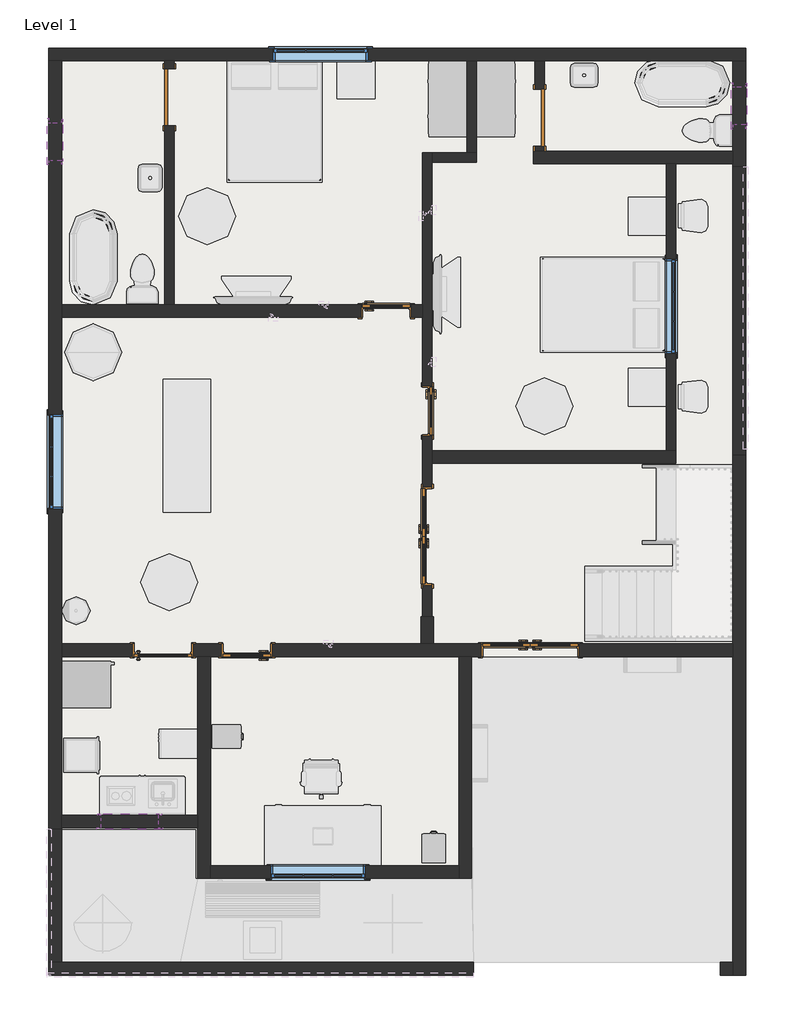
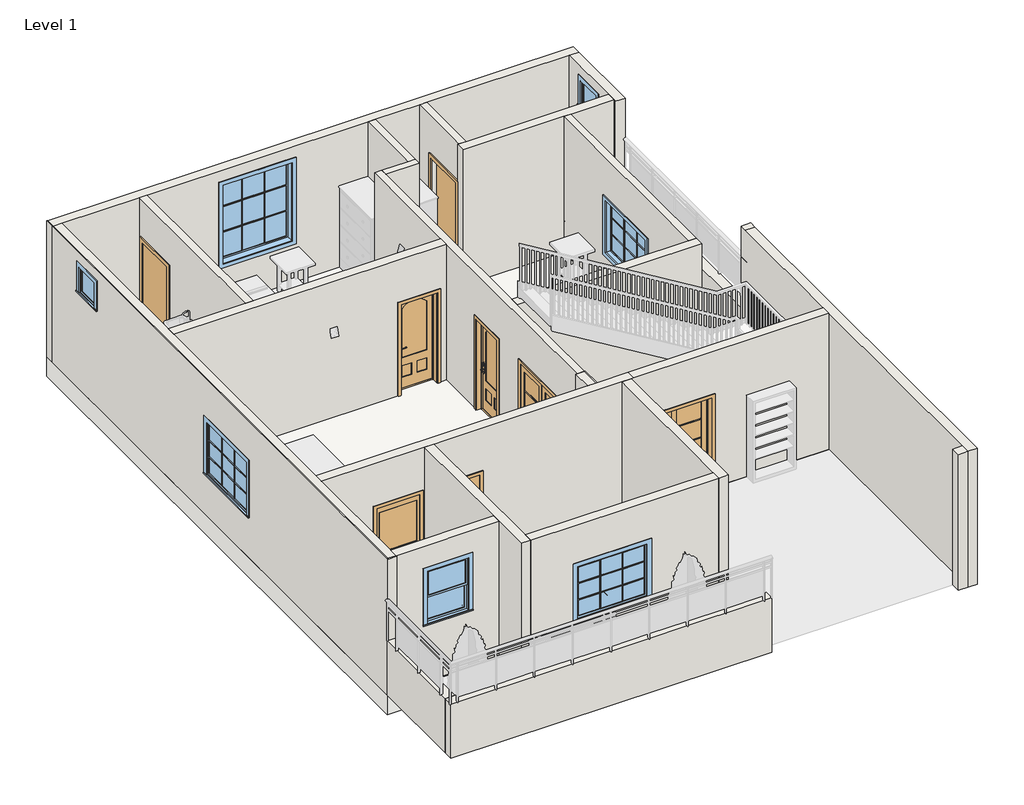
# One storey, part 1 of 4: 23 walls, 8 doors, 7 windows, 1 slab.
"""IFC4 building model written with IfcOpenShell, lengths in millimetres."""

from ifc_helpers import new_model, si_unit, frame, origin, origin_with_axes, place, context, project, spatial, polyline, outline, extrude, faceted_brep, transform, mapped, element, save
from components import door_41326d50, door_4b146b56, door_b03bd389, door_94998e6c, door_30de5629, door_16372e1c, window_a4fe791f, window_1f50baaf, window_cc15f82e, window_31198920, window_e41d21a6

model = new_model("IFC4")

# Units and contexts
model_context = context("Model", 3, world=origin())
ifc_project = project(units=[si_unit("LENGTHUNIT", "METRE", prefix="MILLI")], contexts=[model_context])

# Site, building, storey
site = spatial("IfcSite", under=ifc_project)
building = spatial("IfcBuilding", under=site)
storey = spatial("IfcBuildingStorey", under=building, Name="Level 1", Elevation=0.0)

# Doors
placement = place(None, origin())
door_shape = door_41326d50(model_context)
element("IfcDoor", 1, ObjectType="30\" x 80\"", at=placement, inside=storey, context=model_context, shape_type="MappedRepresentation", body=[
    mapped(door_shape, transform((-6354.9886283, 7720.7324946, 0.0), x_axis=(-1.0, 0.0, 0.0), y_axis=(0.0, -1.0, 0.0), z_axis=(0.0, 0.0, 1.0))),
])
element("IfcDoor", 2, ObjectType="30\" x 80\"", at=placement, inside=storey, context=model_context, shape_type="MappedRepresentation", body=[
    mapped(door_shape, transform((-8590.1886283, 2278.7824946, 0.0), x_axis=(1.0, 0.0, 0.0), y_axis=(0.0, 1.0, 0.0), z_axis=(0.0, 0.0, 1.0))),
])
door_2_shape = door_4b146b56(model_context)
element("IfcDoor", 3, ObjectType="30\" x 80\"", at=placement, inside=storey, context=model_context, shape_type="MappedRepresentation", body=[
    mapped(door_2_shape, transform((-5691.4136283, 6117.3574946, 0.0), x_axis=(0.0, 1.0, 0.0), y_axis=(-1.0, 0.0, 0.0), z_axis=(0.0, 0.0, 1.0))),
])
door_3_shape = door_b03bd389(model_context)
element("IfcDoor", 4, ObjectType="Door-Exterior-Double-Full Glass-Wood_Clad : 60\" x 80\"", at=placement, inside=storey, context=model_context, shape_type="MappedRepresentation", body=[
    mapped(door_3_shape, transform((-4043.5886283, 2285.1324946, 0.0), x_axis=(1.0, 0.0, 0.0), y_axis=(0.0, 1.0, 0.0), z_axis=(0.0, 0.0, 1.0))),
])
door_4_shape = door_94998e6c(model_context)
element("IfcDoor", 5, ObjectType="Door-Exterior-Double-Full Glass-Wood_Clad : 60\" x 80\"", at=placement, inside=storey, context=model_context, shape_type="MappedRepresentation", body=[
    mapped(door_4_shape, transform((-5697.7636283, 4110.7574946, 0.0), x_axis=(0.0, 1.0, 0.0), y_axis=(-1.0, 0.0, 0.0), z_axis=(0.0, 0.0, 1.0))),
])
door_5_shape = door_30de5629(model_context)
element("IfcDoor", 6, ObjectType="Door-Interior-Single-2_Panel-Wood : 36\" x 80\"", at=placement, inside=storey, context=model_context, shape_type="MappedRepresentation", body=[
    mapped(door_5_shape, transform((-9936.3886283, 2278.7824946, 0.0), x_axis=(1.0, 0.0, 0.0), y_axis=(0.0, 1.0, 0.0), z_axis=(0.0, 0.0, 1.0))),
])
door_6_shape = door_16372e1c(model_context)
element("IfcDoor", 7, ObjectType="Single-Flush : 36\" x 84\"", at=placement, inside=storey, context=model_context, shape_type="MappedRepresentation", body=[
    mapped(door_6_shape, transform((-9834.7886283, 11146.5574946, 0.0), x_axis=(0.0, 1.0, 0.0), y_axis=(-1.0, 0.0, 0.0), z_axis=(0.0, 0.0, 1.0))),
])
element("IfcDoor", 8, ObjectType="Single-Flush : 36\" x 84\"", at=placement, inside=storey, context=model_context, shape_type="MappedRepresentation", body=[
    mapped(door_6_shape, transform((-3891.1886283, 10816.3574946, 0.0), x_axis=(0.0, -1.0, 0.0), y_axis=(1.0, 0.0, 0.0), z_axis=(0.0, 0.0, 1.0))),
])

# Slab
element("IfcSlab", 9, ObjectType="Steel Bar Joist 14\" - VCT on Concrete", at=placement, inside=storey, context=model_context, shape_type="SweptSolid", body=[
    extrude(outline(polyline([(-11765.1886283, -588.2425054), (-11765.1886283, 11933.9574946), (-589.1886283, 11933.9574946), (-589.1886283, 2180.3574946), (-4983.3886283, 2180.3574946), (-4983.3886283, -1375.6425054), (-9402.9886283, -1375.6425054), (-9402.9886283, -588.2425054), (-11765.1886283, -588.2425054)])), frame((0.0, 0.0, -441.325), z_axis=(0.0, 0.0, 1.0), x_axis=(1.0, 0.0, 0.0)), (0.0, 0.0, 1.0), 441.325),
])

# Walls
element("IfcWall", 10, ObjectType="Generic - 8\"", at=placement, inside=storey, context=model_context, shape_type="Brep", body=[
    faceted_brep([(-11765.1886283, 11730.7574946, 0.0), (-11561.9886283, 11730.7574946, 0.0), (-9910.9886283, 11730.7574946, 0.0), (-9758.5886283, 11730.7574946, 0.0), (-5059.5886283, 11730.7574946, 0.0), (-4907.1886283, 11730.7574946, 0.0), (-3967.3886283, 11730.7574946, 0.0), (-3814.9886283, 11730.7574946, 0.0), (-792.3886283, 11730.7574946, 0.0), (-589.1886283, 11730.7574946, 0.0), (-589.1886283, 11730.7574946, 3048.0), (-792.3886283, 11730.7574946, 3048.0), (-3814.9886283, 11730.7574946, 3048.0), (-3967.3886283, 11730.7574946, 3048.0), (-4907.1886283, 11730.7574946, 3048.0), (-5059.5886283, 11730.7574946, 3048.0), (-9758.5886283, 11730.7574946, 3048.0), (-9910.9886283, 11730.7574946, 3048.0), (-11561.9886283, 11730.7574946, 3048.0), (-11739.7886283, 11730.7574946, 3048.0), (-11765.1886283, 11730.7574946, 3048.0), (-6647.0886283, 11730.7574946, 2743.2), (-6647.0886283, 11730.7574946, 914.4), (-8171.0886283, 11730.7574946, 914.4), (-8171.0886283, 11730.7574946, 2743.2), (-11765.1886283, 11933.9574946, 0.0), (-11765.1886283, 11933.9574946, 3048.0), (-11739.7886283, 11933.9574946, 3048.0), (-589.1886283, 11933.9574946, 3048.0), (-589.1886283, 11933.9574946, 0.0), (-6647.0886283, 11933.9574946, 2743.2), (-8171.0886283, 11933.9574946, 2743.2), (-8171.0886283, 11933.9574946, 914.4), (-6647.0886283, 11933.9574946, 914.4)], [[[0, 1, 2, 3, 4, 5, 6, 7, 8, 9, 10, 11, 12, 13, 14, 15, 16, 17, 18, 19, 20], [21, 22, 23, 24]], [[25, 26, 27, 28, 29], [30, 31, 32, 33]], [[9, 8, 7, 6, 5, 4, 3, 2, 1, 0, 25, 29]], [[10, 9, 29, 28]], [[0, 20, 26, 25]], [[22, 21, 30, 33]], [[23, 22, 33, 32]], [[24, 23, 32, 31]], [[21, 24, 31, 30]], [[20, 19, 27, 26]], [[19, 18, 17, 16, 15, 14, 13, 12, 11, 10, 28, 27]]]),
])
element("IfcWall", 11, ObjectType="Generic - 8\"", at=placement, inside=storey, context=model_context, shape_type="Brep", body=[
    faceted_brep([(-792.3886283, 11730.7574946, 0.0), (-792.3886283, 10282.9574946, 0.0), (-792.3886283, 10079.7574946, 0.0), (-792.3886283, 10028.9574946, 0.0), (-792.3886283, 10028.9574946, 1219.2), (-792.3886283, 10028.9574946, 3048.0), (-792.3886283, 10079.7574946, 3048.0), (-792.3886283, 10282.9574946, 3048.0), (-792.3886283, 11730.7574946, 3048.0), (-792.3886283, 11311.6574946, 2768.6), (-792.3886283, 10702.0574946, 2768.6), (-792.3886283, 10702.0574946, 2159.0), (-792.3886283, 11311.6574946, 2159.0), (-589.1886283, 11730.7574946, 0.0), (-589.1886283, 11730.7574946, 3048.0), (-589.1886283, 10028.9574946, 3048.0), (-589.1886283, 10028.9574946, 1219.2), (-589.1886283, 10028.9574946, 0.0), (-589.1886283, 11311.6574946, 2768.6), (-589.1886283, 11311.6574946, 2159.0), (-589.1886283, 10702.0574946, 2159.0), (-589.1886283, 10702.0574946, 2768.6)], [[[0, 1, 2, 3, 4, 5, 6, 7, 8], [9, 10, 11, 12]], [[13, 14, 15, 16, 17], [18, 19, 20, 21]], [[3, 2, 1, 0, 13, 17]], [[5, 4, 3, 17, 16, 15]], [[0, 8, 14, 13]], [[19, 18, 9, 12]], [[20, 19, 12, 11]], [[21, 20, 11, 10]], [[18, 21, 10, 9]], [[8, 7, 6, 5, 15, 14]]]),
])
element("IfcWall", 12, ObjectType="Generic - 8\"", at=placement, inside=storey, context=model_context, shape_type="SweptSolid", body=[
    extrude(outline(polyline([(-995.5886283, -2721.8425054), (-792.3886283, -2721.8425054), (-792.3886283, -2925.0425054), (-995.5886283, -2925.0425054), (-995.5886283, -2721.8425054)])), origin_with_axes(), (0.0, 0.0, 1.0), 3048.0),
])
element("IfcWall", 13, ObjectType="Generic - 8\"", at=placement, inside=storey, context=model_context, shape_type="SweptSolid", body=[
    extrude(outline(polyline([(-11561.9886283, -588.2425054), (-11561.9886283, -2721.8425054), (-11765.1886283, -2721.8425054), (-11765.1886283, -588.2425054), (-11561.9886283, -588.2425054)])), origin_with_axes(), (0.0, 0.0, 1.0), 1219.2),
])
element("IfcWall", 14, ObjectType="Generic - 8\"", at=placement, inside=storey, context=model_context, shape_type="Brep", body=[
    faceted_brep([(-11561.9886283, 7615.9574946, 3048.0), (-11561.9886283, 7615.9574946, 0.0), (-6761.3886283, 7615.9574946, 0.0), (-6761.3886283, 7615.9574946, 2057.4), (-5948.5886283, 7615.9574946, 2057.4), (-5948.5886283, 7615.9574946, 0.0), (-5770.7886283, 7615.9574946, 0.0), (-5770.7886283, 7615.9574946, 3048.0), (-11561.9886283, 7819.1574946, 0.0), (-11561.9886283, 7819.1574946, 3048.0), (-9910.9886283, 7819.1574946, 3048.0), (-9758.5886283, 7819.1574946, 3048.0), (-5770.7886283, 7819.1574946, 3048.0), (-5770.7886283, 7819.1574946, 0.0), (-5948.5886283, 7819.1574946, 0.0), (-5948.5886283, 7819.1574946, 2057.4), (-6761.3886283, 7819.1574946, 2057.4), (-6761.3886283, 7819.1574946, 0.0), (-9758.5886283, 7819.1574946, 0.0), (-9910.9886283, 7819.1574946, 0.0)], [[[0, 1, 2, 3, 4, 5, 6, 7]], [[8, 9, 10, 11, 12, 13, 14, 15, 16, 17, 18, 19]], [[1, 8, 19, 18, 17, 2]], [[13, 6, 5, 14]], [[1, 0, 9, 8]], [[7, 6, 13, 12]], [[16, 3, 2, 17]], [[3, 16, 15, 4]], [[4, 15, 14, 5]], [[0, 7, 12, 11, 10, 9]]]),
])
element("IfcWall", 15, ObjectType="Generic - 8\"", at=placement, inside=storey, context=model_context, shape_type="Brep", body=[
    faceted_brep([(-5592.9886283, 2383.5574946, 0.0), (-5592.9886283, 2815.3574946, 0.0), (-5592.9886283, 2815.3574946, 3048.0), (-5592.9886283, 2383.5574946, 3048.0), (-5796.1886283, 2383.5574946, 0.0), (-5796.1886283, 2383.5574946, 3048.0), (-5796.1886283, 2815.3574946, 3048.0), (-5796.1886283, 2815.3574946, 0.0), (-5770.7886283, 2815.3574946, 0.0), (-5618.3886283, 2815.3574946, 0.0), (-5770.7886283, 2815.3574946, 3048.0), (-5618.3886283, 2815.3574946, 3048.0), (-5618.3886283, 2383.5574946, 3048.0), (-5618.3886283, 2408.9574946, 3048.0)], [[[0, 1, 2, 3]], [[4, 5, 6, 7]], [[1, 0, 4, 7, 8, 9]], [[2, 1, 9, 8, 7, 6, 10, 11]], [[0, 3, 12, 5, 4]], [[3, 2, 11, 13, 12]], [[11, 10, 6, 5, 12, 13]]]),
])
element("IfcWall", 16, ObjectType="Generic - 8\"", at=placement, inside=storey, context=model_context, shape_type="Brep", body=[
    faceted_brep([(-792.3886283, 2383.5574946, 3048.0), (-792.3886283, 2383.5574946, 0.0), (-3256.1886283, 2383.5574946, 0.0), (-3256.1886283, 2383.5574946, 2057.4), (-4830.9886283, 2383.5574946, 2057.4), (-4830.9886283, 2383.5574946, 0.0), (-5592.9886283, 2383.5574946, 0.0), (-5796.1886283, 2383.5574946, 0.0), (-8183.7886283, 2383.5574946, 0.0), (-8183.7886283, 2383.5574946, 2057.4), (-8996.5886283, 2383.5574946, 2057.4), (-8996.5886283, 2383.5574946, 0.0), (-9453.7886283, 2383.5574946, 0.0), (-9453.7886283, 2383.5574946, 2057.4), (-10418.9886283, 2383.5574946, 2057.4), (-10418.9886283, 2383.5574946, 0.0), (-11561.9886283, 2383.5574946, 0.0), (-11561.9886283, 2383.5574946, 3048.0), (-5796.1886283, 2383.5574946, 3048.0), (-5592.9886283, 2383.5574946, 3048.0), (-4932.5886283, 2383.5574946, 3048.0), (-792.3886283, 2180.3574946, 0.0), (-792.3886283, 2180.3574946, 3048.0), (-4932.5886283, 2180.3574946, 3048.0), (-4983.3886283, 2180.3574946, 3048.0), (-5186.5886283, 2180.3574946, 3048.0), (-9174.3886283, 2180.3574946, 3048.0), (-9377.5886283, 2180.3574946, 3048.0), (-11561.9886283, 2180.3574946, 3048.0), (-11561.9886283, 2180.3574946, 0.0), (-10418.9886283, 2180.3574946, 0.0), (-10418.9886283, 2180.3574946, 2057.4), (-9453.7886283, 2180.3574946, 2057.4), (-9453.7886283, 2180.3574946, 0.0), (-9377.5886283, 2180.3574946, 0.0), (-9174.3886283, 2180.3574946, 0.0), (-8996.5886283, 2180.3574946, 0.0), (-8996.5886283, 2180.3574946, 2057.4), (-8183.7886283, 2180.3574946, 2057.4), (-8183.7886283, 2180.3574946, 0.0), (-5186.5886283, 2180.3574946, 0.0), (-4983.3886283, 2180.3574946, 0.0), (-4830.9886283, 2180.3574946, 0.0), (-4830.9886283, 2180.3574946, 2057.4), (-3256.1886283, 2180.3574946, 2057.4), (-3256.1886283, 2180.3574946, 0.0)], [[[0, 1, 2, 3, 4, 5, 6, 7, 8, 9, 10, 11, 12, 13, 14, 15, 16, 17, 18, 19, 20]], [[21, 22, 23, 24, 25, 26, 27, 28, 29, 30, 31, 32, 33, 34, 35, 36, 37, 38, 39, 40, 41, 42, 43, 44, 45]], [[1, 21, 45, 2]], [[29, 16, 15, 30]], [[5, 42, 41, 40, 39, 8, 7, 6]], [[33, 12, 11, 36, 35, 34]], [[1, 0, 22, 21]], [[17, 16, 29, 28]], [[44, 3, 2, 45]], [[3, 44, 43, 4]], [[4, 43, 42, 5]], [[32, 13, 12, 33]], [[13, 32, 31, 14]], [[14, 31, 30, 15]], [[38, 9, 8, 39]], [[9, 38, 37, 10]], [[10, 37, 36, 11]], [[22, 0, 20, 23]], [[20, 19, 18, 17, 28, 27, 26, 25, 24, 23]]]),
])
element("IfcWall", 17, ObjectType="Generic - 8\"", at=placement, inside=storey, context=model_context, shape_type="Brep", body=[
    faceted_brep([(-9377.5886283, 2180.3574946, 0.0), (-9377.5886283, -359.6425054, 0.0), (-9377.5886283, -562.8425054, 0.0), (-9377.5886283, -1375.6425054, 0.0), (-9377.5886283, -1375.6425054, 3048.0), (-9377.5886283, -562.8425054, 3048.0), (-9377.5886283, -359.6425054, 3048.0), (-9377.5886283, 2180.3574946, 3048.0), (-9174.3886283, 2180.3574946, 0.0), (-9174.3886283, 2180.3574946, 3048.0), (-9174.3886283, -1172.4425054, 3048.0), (-9174.3886283, -1375.6425054, 3048.0), (-9174.3886283, -1375.6425054, 0.0), (-9174.3886283, -1172.4425054, 0.0)], [[[0, 1, 2, 3, 4, 5, 6, 7]], [[8, 9, 10, 11, 12, 13]], [[3, 2, 1, 0, 8, 13, 12]], [[0, 7, 9, 8]], [[4, 3, 12, 11]], [[7, 6, 5, 4, 11, 10, 9]]]),
])
element("IfcWall", 18, ObjectType="Generic - 8\"", at=placement, inside=storey, context=model_context, shape_type="SweptSolid", body=[
    extrude(outline(polyline([(0.0, -9174.3886283), (0.0, -5186.5886283), (3048.0, -5186.5886283), (3048.0, -9174.3886283), (0.0, -9174.3886283)]), holes=[polyline([(2133.6, -8209.1886283), (2133.6, -6685.1886283), (914.4, -6685.1886283), (914.4, -8209.1886283), (2133.6, -8209.1886283)])]), frame((0.0, -1375.6425054, 0.0), z_axis=(0.0, 1.0, 0.0), x_axis=(0.0, 0.0, 1.0)), (0.0, 0.0, 1.0), 203.2),
])
element("IfcWall", 19, ObjectType="Generic - 8\"", at=placement, inside=storey, context=model_context, shape_type="SweptSolid", body=[
    extrude(outline(polyline([(0.0, -9377.5886283), (3048.0, -9377.5886283), (3048.0, -11561.9886283), (0.0, -11561.9886283), (0.0, -9377.5886283)]), holes=[polyline([(2489.2, -10926.9886283), (2489.2, -10012.5886283), (1270.0, -10012.5886283), (1270.0, -10926.9886283), (2489.2, -10926.9886283)])]), frame((0.0, -562.8425054, 0.0), z_axis=(0.0, 1.0, 0.0), x_axis=(0.0, 0.0, 1.0)), (0.0, 0.0, 1.0), 203.2),
])
element("IfcWall", 20, ObjectType="Generic - 8\"", at=placement, inside=storey, context=model_context, shape_type="Brep", body=[
    faceted_brep([(-4957.9886283, -2721.8425054, 0.0), (-11561.9886283, -2721.8425054, 0.0), (-11765.1886283, -2721.8425054, 0.0), (-11765.1886283, -2721.8425054, 1219.2), (-11561.9886283, -2721.8425054, 1219.2), (-4957.9886283, -2721.8425054, 1219.2), (-4957.9886283, -2925.0425054, 0.0), (-4957.9886283, -2925.0425054, 1219.2), (-11765.1886283, -2925.0425054, 1219.2), (-11765.1886283, -2925.0425054, 0.0)], [[[0, 1, 2, 3, 4, 5]], [[6, 7, 8, 9]], [[2, 1, 0, 6, 9]], [[5, 4, 3, 8, 7]], [[0, 5, 7, 6]], [[3, 2, 9, 8]]]),
])
element("IfcWall", 21, ObjectType="Generic - 8\"", at=placement, inside=storey, context=model_context, shape_type="Brep", body=[
    faceted_brep([(-4983.3886283, -1375.6425054, 0.0), (-4983.3886283, 2180.3574946, 0.0), (-4983.3886283, 2180.3574946, 3048.0), (-4983.3886283, -1375.6425054, 3048.0), (-5186.5886283, -1375.6425054, 0.0), (-5186.5886283, -1375.6425054, 3048.0), (-5186.5886283, -1172.4425054, 3048.0), (-5186.5886283, 2180.3574946, 3048.0), (-5186.5886283, 2180.3574946, 0.0), (-5186.5886283, -1172.4425054, 0.0)], [[[0, 1, 2, 3]], [[4, 5, 6, 7, 8, 9]], [[1, 0, 4, 9, 8]], [[2, 1, 8, 7]], [[0, 3, 5, 4]], [[3, 2, 7, 6, 5]]]),
])
element("IfcWall", 22, ObjectType="Generic - 8\"", at=placement, inside=storey, context=model_context, shape_type="Brep", body=[
    faceted_brep([(-11561.9886283, -588.2425054, 0.0), (-11561.9886283, -562.8425054, 0.0), (-11561.9886283, -359.6425054, 0.0), (-11561.9886283, 2180.3574946, 0.0), (-11561.9886283, 2383.5574946, 0.0), (-11561.9886283, 7615.9574946, 0.0), (-11561.9886283, 7819.1574946, 0.0), (-11561.9886283, 11730.7574946, 0.0), (-11561.9886283, 11730.7574946, 3048.0), (-11561.9886283, 7819.1574946, 3048.0), (-11561.9886283, 7615.9574946, 3048.0), (-11561.9886283, 2383.5574946, 3048.0), (-11561.9886283, 2180.3574946, 3048.0), (-11561.9886283, -359.6425054, 3048.0), (-11561.9886283, -562.8425054, 3048.0), (-11561.9886283, -588.2425054, 3048.0), (-11561.9886283, -588.2425054, 1219.2), (-11561.9886283, 6066.5574946, 2133.6), (-11561.9886283, 6066.5574946, 914.4), (-11561.9886283, 4542.5574946, 914.4), (-11561.9886283, 4542.5574946, 2133.6), (-11561.9886283, 10740.1574946, 2768.6), (-11561.9886283, 10740.1574946, 2159.0), (-11561.9886283, 10130.5574946, 2159.0), (-11561.9886283, 10130.5574946, 2768.6), (-11765.1886283, -588.2425054, 0.0), (-11765.1886283, -588.2425054, 1219.2), (-11765.1886283, -588.2425054, 3048.0), (-11765.1886283, -562.8425054, 3048.0), (-11765.1886283, 11730.7574946, 3048.0), (-11765.1886283, 11730.7574946, 0.0), (-11765.1886283, 6066.5574946, 2133.6), (-11765.1886283, 4542.5574946, 2133.6), (-11765.1886283, 4542.5574946, 914.4), (-11765.1886283, 6066.5574946, 914.4), (-11765.1886283, 10740.1574946, 2768.6), (-11765.1886283, 10130.5574946, 2768.6), (-11765.1886283, 10130.5574946, 2159.0), (-11765.1886283, 10740.1574946, 2159.0), (-11739.7886283, -588.2425054, 3048.0), (-11739.7886283, 11730.7574946, 3048.0), (-11739.7886283, -562.8425054, 3048.0)], [[[0, 1, 2, 3, 4, 5, 6, 7, 8, 9, 10, 11, 12, 13, 14, 15, 16], [17, 18, 19, 20], [21, 22, 23, 24]], [[25, 26, 27, 28, 29, 30], [31, 32, 33, 34], [35, 36, 37, 38]], [[7, 6, 5, 4, 3, 2, 1, 0, 25, 30]], [[0, 16, 15, 39, 27, 26, 25]], [[8, 7, 30, 29, 40]], [[18, 17, 31, 34]], [[19, 18, 34, 33]], [[20, 19, 33, 32]], [[17, 20, 32, 31]], [[22, 21, 35, 38]], [[23, 22, 38, 37]], [[24, 23, 37, 36]], [[21, 24, 36, 35]], [[40, 29, 28, 41]], [[15, 14, 41, 39]], [[41, 28, 27, 39]], [[14, 13, 12, 11, 10, 9, 8, 40, 41]]]),
])
element("IfcWall", 23, ObjectType="Generic - 8\"", at=placement, inside=storey, context=model_context, shape_type="SweptSolid", body=[
    extrude(outline(polyline([(-792.3886283, 5406.1574946), (-792.3886283, 10028.9574946), (-589.1886283, 10028.9574946), (-589.1886283, 5406.1574946), (-792.3886283, 5406.1574946)])), origin_with_axes(), (0.0, 0.0, 1.0), 1219.2),
])
element("IfcWall", 24, ObjectType="Generic - 8\"", at=placement, inside=storey, context=model_context, shape_type="Brep", body=[
    faceted_brep([(-792.3886283, 5406.1574946, 0.0), (-792.3886283, 2383.5574946, 0.0), (-792.3886283, 2180.3574946, 0.0), (-792.3886283, -2721.8425054, 0.0), (-792.3886283, -2925.0425054, 0.0), (-792.3886283, -2925.0425054, 3048.0), (-792.3886283, -2721.8425054, 3048.0), (-792.3886283, 2180.3574946, 3048.0), (-792.3886283, 2383.5574946, 3048.0), (-792.3886283, 5253.7574946, 3048.0), (-792.3886283, 5406.1574946, 3048.0), (-792.3886283, 5406.1574946, 1219.2), (-589.1886283, 5406.1574946, 0.0), (-589.1886283, 5406.1574946, 1219.2), (-589.1886283, 5406.1574946, 3048.0), (-589.1886283, 5253.7574946, 3048.0), (-589.1886283, -2925.0425054, 3048.0), (-589.1886283, -2925.0425054, 0.0)], [[[0, 1, 2, 3, 4, 5, 6, 7, 8, 9, 10, 11]], [[12, 13, 14, 15, 16, 17]], [[4, 3, 2, 1, 0, 12, 17]], [[0, 11, 10, 14, 13, 12]], [[5, 4, 17, 16]], [[9, 8, 7, 6, 5, 16, 15]], [[10, 9, 15, 14]]]),
])
element("IfcWall", 25, ObjectType="Generic - 8\"", at=placement, inside=storey, context=model_context, shape_type="Brep", body=[
    faceted_brep([(-1706.7886283, 5482.3574946, 0.0), (-1859.1886283, 5482.3574946, 0.0), (-5618.3886283, 5482.3574946, 0.0), (-5618.3886283, 5482.3574946, 3048.0), (-1859.1886283, 5482.3574946, 3048.0), (-1706.7886283, 5482.3574946, 3048.0), (-1706.7886283, 5279.1574946, 0.0), (-1706.7886283, 5279.1574946, 3048.0), (-5618.3886283, 5279.1574946, 3048.0), (-5618.3886283, 5279.1574946, 0.0)], [[[0, 1, 2, 3, 4, 5]], [[6, 7, 8, 9]], [[2, 1, 0, 6, 9]], [[3, 2, 9, 8]], [[0, 5, 7, 6]], [[5, 4, 3, 8, 7]]]),
])
element("IfcWall", 26, ObjectType="Generic - 8\"", at=placement, inside=storey, context=model_context, shape_type="Brep", body=[
    faceted_brep([(-3992.7886283, 10079.7574946, 0.0), (-1859.1886283, 10079.7574946, 0.0), (-1706.7886283, 10079.7574946, 0.0), (-792.3886283, 10079.7574946, 0.0), (-792.3886283, 10079.7574946, 3048.0), (-1706.7886283, 10079.7574946, 3048.0), (-1859.1886283, 10079.7574946, 3048.0), (-3992.7886283, 10079.7574946, 3048.0), (-3992.7886283, 10282.9574946, 0.0), (-3992.7886283, 10282.9574946, 3048.0), (-3967.3886283, 10282.9574946, 3048.0), (-3814.9886283, 10282.9574946, 3048.0), (-792.3886283, 10282.9574946, 3048.0), (-792.3886283, 10282.9574946, 0.0), (-3814.9886283, 10282.9574946, 0.0), (-3967.3886283, 10282.9574946, 0.0)], [[[0, 1, 2, 3, 4, 5, 6, 7]], [[8, 9, 10, 11, 12, 13, 14, 15]], [[3, 2, 1, 0, 8, 15, 14, 13]], [[0, 7, 9, 8]], [[4, 3, 13, 12]], [[7, 6, 5, 4, 12, 11, 10, 9]]]),
])
element("IfcWall", 27, ObjectType="INNER WALL", at=placement, inside=storey, context=model_context, shape_type="Brep", body=[
    faceted_brep([(-5618.3886283, 10105.1574946, 0.0), (-4907.1886283, 10105.1574946, 0.0), (-4907.1886283, 10105.1574946, 3048.0), (-5618.3886283, 10105.1574946, 3048.0), (-5618.3886283, 10257.5574946, 0.0), (-5618.3886283, 10257.5574946, 3048.0), (-5059.5886283, 10257.5574946, 3048.0), (-4907.1886283, 10257.5574946, 3048.0), (-4907.1886283, 10257.5574946, 0.0), (-5059.5886283, 10257.5574946, 0.0)], [[[0, 1, 2, 3]], [[4, 5, 6, 7, 8, 9]], [[1, 0, 4, 9, 8]], [[0, 3, 5, 4]], [[2, 1, 8, 7]], [[3, 2, 7, 6, 5]]]),
])
element("IfcWall", 28, ObjectType="INNER WALL", at=placement, inside=storey, context=model_context, shape_type="SweptSolid", body=[
    extrude(outline(polyline([(10359.1574946, 2133.6), (10359.1574946, 0.0), (10282.9574946, 0.0), (10282.9574946, 3048.0), (11730.7574946, 3048.0), (11730.7574946, 0.0), (11273.5574946, 0.0), (11273.5574946, 2133.6), (10359.1574946, 2133.6)])), frame((-3967.3886283, 0.0, 0.0), z_axis=(1.0, 0.0, 0.0), x_axis=(0.0, 1.0, 0.0)), (0.0, 0.0, 1.0), 152.4),
])
element("IfcWall", 29, ObjectType="INNER WALL", at=placement, inside=storey, context=model_context, shape_type="SweptSolid", body=[
    extrude(outline(polyline([(10079.7574946, 0.0), (5482.3574946, 0.0), (5482.3574946, 3048.0), (10079.7574946, 3048.0), (10079.7574946, 0.0)]), holes=[polyline([(7031.7574946, 2133.6), (7031.7574946, 914.4), (8555.7574946, 914.4), (8555.7574946, 2133.6), (7031.7574946, 2133.6)])]), frame((-1859.1886283, 0.0, 0.0), z_axis=(1.0, 0.0, 0.0), x_axis=(0.0, 1.0, 0.0)), (0.0, 0.0, 1.0), 152.4),
])
element("IfcWall", 30, ObjectType="INNER WALL", at=placement, inside=storey, context=model_context, shape_type="SweptSolid", body=[
    extrude(outline(polyline([(11730.7574946, 0.0), (11603.7574946, 0.0), (11603.7574946, 2133.6), (10689.3574946, 2133.6), (10689.3574946, 0.0), (7819.1574946, 0.0), (7819.1574946, 3048.0), (11730.7574946, 3048.0), (11730.7574946, 0.0)])), frame((-9910.9886283, 0.0, 0.0), z_axis=(1.0, 0.0, 0.0), x_axis=(0.0, 1.0, 0.0)), (0.0, 0.0, 1.0), 152.4),
])
element("IfcWall", 31, ObjectType="INNER WALL", at=placement, inside=storey, context=model_context, shape_type="Brep", body=[
    faceted_brep([(-5618.3886283, 2815.3574946, 3048.0), (-5618.3886283, 2815.3574946, 0.0), (-5618.3886283, 3323.3574946, 0.0), (-5618.3886283, 3323.3574946, 2057.4), (-5618.3886283, 4898.1574946, 2057.4), (-5618.3886283, 4898.1574946, 0.0), (-5618.3886283, 5279.1574946, 0.0), (-5618.3886283, 5482.3574946, 0.0), (-5618.3886283, 5710.9574946, 0.0), (-5618.3886283, 5710.9574946, 2057.4), (-5618.3886283, 6523.7574946, 2057.4), (-5618.3886283, 6523.7574946, 0.0), (-5618.3886283, 10105.1574946, 0.0), (-5618.3886283, 10257.5574946, 0.0), (-5618.3886283, 10257.5574946, 3048.0), (-5618.3886283, 10105.1574946, 3048.0), (-5618.3886283, 5482.3574946, 3048.0), (-5618.3886283, 5279.1574946, 3048.0), (-5618.3886283, 5253.7574946, 3048.0), (-5770.7886283, 2815.3574946, 3048.0), (-5770.7886283, 7615.9574946, 3048.0), (-5770.7886283, 7819.1574946, 3048.0), (-5770.7886283, 10257.5574946, 3048.0), (-5770.7886283, 10257.5574946, 0.0), (-5770.7886283, 7819.1574946, 0.0), (-5770.7886283, 7615.9574946, 0.0), (-5770.7886283, 6523.7574946, 0.0), (-5770.7886283, 6523.7574946, 2057.4), (-5770.7886283, 5710.9574946, 2057.4), (-5770.7886283, 5710.9574946, 0.0), (-5770.7886283, 4898.1574946, 0.0), (-5770.7886283, 4898.1574946, 2057.4), (-5770.7886283, 3323.3574946, 2057.4), (-5770.7886283, 3323.3574946, 0.0), (-5770.7886283, 2815.3574946, 0.0)], [[[0, 1, 2, 3, 4, 5, 6, 7, 8, 9, 10, 11, 12, 13, 14, 15, 16, 17, 18]], [[19, 20, 21, 22, 23, 24, 25, 26, 27, 28, 29, 30, 31, 32, 33, 34]], [[1, 34, 33, 2]], [[23, 13, 12, 11, 26, 25, 24]], [[5, 30, 29, 8, 7, 6]], [[1, 0, 19, 34]], [[14, 13, 23, 22]], [[4, 31, 30, 5]], [[31, 4, 3, 32]], [[32, 3, 2, 33]], [[10, 27, 26, 11]], [[27, 10, 9, 28]], [[28, 9, 8, 29]], [[22, 21, 20, 19, 0, 18, 17, 16, 15, 14]]]),
])
element("IfcWall", 32, ObjectType="INNER WALL", at=placement, inside=storey, context=model_context, shape_type="SweptSolid", body=[
    extrude(outline(polyline([(-5059.5886283, 10257.5574946), (-5059.5886283, 11730.7574946), (-4907.1886283, 11730.7574946), (-4907.1886283, 10257.5574946), (-5059.5886283, 10257.5574946)])), origin_with_axes(), (0.0, 0.0, 1.0), 3048.0),
])

# Windows
window_shape = window_a4fe791f(model_context)
element("IfcWindow", 33, ObjectType="Casement 3x3 with Trim : 60\" x 48\"", at=placement, inside=storey, context=model_context, shape_type="MappedRepresentation", body=[
    mapped(window_shape, transform((-7447.1886283, -1274.0425054, 0.0), x_axis=(-1.0, 0.0, 0.0), y_axis=(0.0, -1.0, 0.0), z_axis=(0.0, 0.0, 1.0))),
])
element("IfcWindow", 34, ObjectType="Casement 3x3 with Trim : 60\" x 48\"", at=placement, inside=storey, context=model_context, shape_type="MappedRepresentation", body=[
    mapped(window_shape, transform((-11663.5886283, 5304.5574946, 0.0), x_axis=(0.0, 1.0, 0.0), y_axis=(-1.0, 0.0, 0.0), z_axis=(0.0, 0.0, 1.0))),
])
window_2_shape = window_1f50baaf(model_context)
element("IfcWindow", 35, ObjectType="Casement 3x3 with Trim : 60\" x 48\"", at=placement, inside=storey, context=model_context, shape_type="MappedRepresentation", body=[
    mapped(window_2_shape, transform((-1782.9886283, 7793.7574946, 0.0), x_axis=(0.0, -1.0, 0.0), y_axis=(1.0, 0.0, 0.0), z_axis=(0.0, 0.0, 1.0))),
])
window_3_shape = window_cc15f82e(model_context)
element("IfcWindow", 36, ObjectType="Casement 3x3 with Trim : 60\" x 72\"", at=placement, inside=storey, context=model_context, shape_type="MappedRepresentation", body=[
    mapped(window_3_shape, transform((-7409.0886283, 11832.3574946, 609.6), x_axis=(1.0, 0.0, 0.0), y_axis=(0.0, 1.0, 0.0), z_axis=(0.0, 0.0, 1.0))),
])
window_4_shape = window_31198920(model_context)
element("IfcWindow", 37, ObjectType="Double Hung with Trim : 36\" x 48\"", at=placement, inside=storey, context=model_context, shape_type="MappedRepresentation", body=[
    mapped(window_4_shape, transform((-10469.7886283, -461.2425054, 355.6), x_axis=(-1.0, 0.0, 0.0), y_axis=(0.0, -1.0, 0.0), z_axis=(0.0, 0.0, 1.0))),
])
window_5_shape = window_e41d21a6(model_context)
element("IfcWindow", 38, ObjectType="Transom with Trim : 24\" x 24\"", at=placement, inside=storey, context=model_context, shape_type="MappedRepresentation", body=[
    mapped(window_5_shape, transform((-690.7886283, 11044.9574946, 0.0), x_axis=(0.0, 1.0, 0.0), y_axis=(-1.0, 0.0, 0.0), z_axis=(0.0, 0.0, 1.0))),
])
element("IfcWindow", 39, ObjectType="Transom with Trim : 24\" x 24\"", at=placement, inside=storey, context=model_context, shape_type="MappedRepresentation", body=[
    mapped(window_5_shape, transform((-11663.5886283, 10473.4574946, 0.0), x_axis=(0.0, 1.0, 0.0), y_axis=(-1.0, 0.0, 0.0), z_axis=(0.0, 0.0, 1.0))),
])

save(model, "model.ifc")

# Revit data of these elements
# Type "30\" x 80\""
#   Type Mark = "9"
#   Assembly Code = "B2030100"
#   Analytic Construction = "French door, wood frame with single glass"
#   Threshold Offset [instance default] = 0' - 0 1/2"
#   Thickness = 0' - 1 3/8"
#   Thermal Resistance (R) = 1.0696 (h·ft²·°F)/BTU
#   Swing Angle [instance default] = 90.00°
#   Stiles = 0' - 4 3/4"
#   Rough Width = 2' - 8"
#   Rough Height = 6' - 9"
#   Radius = 1' - 1.00625"
#   Lock Rail = 0' - 7 1/8"
#   Height = 6' - 8"
#   Width = 2' - 6"
#   Heat Transfer Coefficient (U) = 0.9350 BTU/(h·ft²·°F)
#   Door Offset [instance default] = 0' - 0"
#   Bottom Rail = 0' - 9 1/2"
#   Threshold [instance default] = yes
#   Function = 1
#   Exterior Trim [instance default] = yes
#   Trim Material = Cherry
#   Threshold Material = Cherry
#   Panel Material = Cherry
#   Glazing = Glass
#   Frame Material = Cherry
#   Door Handle Material = Aluminum
#   Visual Light Transmittance = 0
#   Solar Heat Gain Coefficient = 0
#   Wall Closure = (empty or 0)
#   Construction Type = (empty or 0)
# Type "Door-Exterior-Double-Full Glass-Wood_Clad : 60\" x 80\""
#   Type Mark = "8"
#   Assembly Code = "B2030100"
#   Analytic Construction = "French door, wood frame with double glass"
#   Top Rail = 0' - 4 11/16"
#   Threshold Offset [instance default] = 0' - 0 1/2"
#   Thickness = 0' - 1 3/8"
#   Thermal Resistance (R) = 1.9158 (h·ft²·°F)/BTU
#   Swing Angle [instance default] = 90.00°
#   Stiles = 0' - 4 3/4"
#   Rough Width = 5' - 2"
#   Rough Height = 6' - 9"
#   Panel Width = 2' - 6"
#   Door Offset [instance default] = 0' - 0"
#   Height = 6' - 8"
#   Width = 5' - 0"
#   Heat Transfer Coefficient (U) = 0.5220 BTU/(h·ft²·°F)
#   Bottom Rail = 0' - 9 1/8"
#   Exterior Trim [instance default] = yes
#   Threshold [instance default] = yes
#   Show Grill [instance default] = yes
#   Function = 1
#   Trim Material = Cherry
#   Threshold Material = Cherry
#   Panel Material = Cherry
#   Glazing = Glass
#   Frame Material = Cherry
#   Door Handle Material = Aluminum
#   Visual Light Transmittance = 0
#   Solar Heat Gain Coefficient = 0
#   Wall Closure = (empty or 0)
#   Construction Type = (empty or 0)
# Type "Door-Interior-Single-2_Panel-Wood : 36\" x 80\""
#   Type Mark = "10"
#   Assembly Code = "C1020300"
#   Analytic Construction = "Wooden"
#   Top Rail = 0' - 4 11/16"
#   Thickness = 0' - 1 3/8"
#   Thermal Resistance (R) = 2.5876 (h·ft²·°F)/BTU
#   Swing Angle [instance default] = 90.00°
#   Stiles = 0' - 2 3/8"
#   Rough Width = 3' - 2"
#   Rough Height = 6' - 9"
#   Lock Rail = 0' - 7 1/2"
#   Height = 6' - 8"
#   Width = 3' - 0"
#   Heat Transfer Coefficient (U) = 0.3865 BTU/(h·ft²·°F)
#   Bottom Rail = 0' - 9 1/8"
#   Trim Material = Cherry
#   Panel Material = Cherry
#   Frame Material = Cherry
#   Door Handle Material = Aluminum
#   Visual Light Transmittance = 0
#   Solar Heat Gain Coefficient = 0
#   Wall Closure = (empty or 0)
#   Function = (empty or 0)
# Type "Single-Flush : 36\" x 84\""
#   Type Mark = "1"
#   Construction Type Id = "MDOOR"
#   Assembly Code = "C1020"
#   Analytic Construction = "Metal"
#   Thickness = 0' - 2"
#   Heat Transfer Coefficient (U) = 0.651978 BTU/(h·ft²·°F)
#   Height = 7' - 0"
#   Trim Projection Ext = 0' - 1"
#   Trim Projection Int = 0' - 1"
#   Trim Width = 0' - 3"
#   Width = 3' - 0"
#   Define Thermal Properties by = 1
#   Door Material = Door - Panel
#   Frame Material = Door - Frame
#   Visual Light Transmittance = 0
#   Solar Heat Gain Coefficient = 0
#   Function = (empty or 0)
#   Wall Closure = (empty or 0)
# Type "Steel Bar Joist 14\" - VCT on Concrete"
#   Assembly Code = "B1010"
#   Function = 0
#   Layers, outside or top first: 0' - 0 1/4" "Vinyl Composition Tile" (function 5); 0' - 3" "Concrete, Lightweight" (function 1); 0' - 0 1/8" "Metal Deck" (function 1); 1' - 2" "Structure, Steel Bar Joist Layer" (function 1)
# Type "Generic - 8\""
#   Assembly Code = "B2010"
#   Layers, outside or top first: 0' - 8" "Brick, Common" (function 1)
# Type "INNER WALL"
#   Assembly Code = "B2010"
#   Layers, outside or top first: 0' - 6" "Brick, Soldier Course" (function 1)
# Type "Casement 3x3 with Trim : 60\" x 48\""
#   Type Mark = "10"
#   Construction Type Id = "GSP4R"
#   Assembly Code = "B2020100"
#   Analytic Construction = "1/8 in Pilkington single glazing"
#   Visual Light Transmittance = 0.9
#   Solar Heat Gain Coefficient = 0.78
#   Heat Transfer Coefficient (U) = 0.6496 BTU/(h·ft²·°F)
#   Height = 4' - 0"
#   Default Sill Height = 3' - 0"
#   Trim Projection - Ext. = 0' - 0 1/2"
#   Trim Projection - Int. = 0' - 0 3/4"
#   Trim Width - Exterior = 0' - 3 1/2"
#   Trim Width - Interior = 0' - 3 1/2"
#   Width = 5' - 0"
#   Window Inset = 0' - 0 3/4"
#   Define Thermal Properties by = 1
#   Glass Pane Material = Glass
#   Sash Material = Sash
#   Trim Exterior Material = Trim
#   Trim Interior Material = Trim
#   Wall Closure = (empty or 0)
# Type "Casement 3x3 with Trim : 60\" x 72\""
#   Type Mark = "12"
#   Construction Type Id = "GSP4R"
#   Assembly Code = "B2020100"
#   Analytic Construction = "1/8 in Pilkington single glazing"
#   Visual Light Transmittance = 0.9
#   Solar Heat Gain Coefficient = 0.78
#   Heat Transfer Coefficient (U) = 0.6496 BTU/(h·ft²·°F)
#   Height = 6' - 0"
#   Default Sill Height = 1' - 0"
#   Trim Projection - Ext. = 0' - 0 1/2"
#   Trim Projection - Int. = 0' - 0 3/4"
#   Trim Width - Exterior = 0' - 3 1/2"
#   Trim Width - Interior = 0' - 3 1/2"
#   Width = 5' - 0"
#   Window Inset = 0' - 0 3/4"
#   Define Thermal Properties by = 1
#   Glass Pane Material = Glass
#   Sash Material = Sash
#   Trim Exterior Material = Trim
#   Trim Interior Material = Trim
#   Wall Closure = (empty or 0)
# Type "Double Hung with Trim : 36\" x 48\""
#   Type Mark = "13"
#   Construction Type Id = "GSP4R"
#   Assembly Code = "B2020100"
#   Analytic Construction = "1/8 in Pilkington single glazing"
#   Visual Light Transmittance = 0.9
#   Solar Heat Gain Coefficient = 0.78
#   Heat Transfer Coefficient (U) = 0.6496 BTU/(h·ft²·°F)
#   Height = 4' - 0"
#   Default Sill Height = 3' - 0"
#   Trim Projection - Ext. = 0' - 0 1/2"
#   Trim Projection - Int. = 0' - 0 3/4"
#   Trim Width - Exterior = 0' - 3 1/2"
#   Trim Width - Interior = 0' - 3 1/2"
#   Width = 3' - 0"
#   Window Inset = 0' - 0 3/4"
#   Define Thermal Properties by = 1
#   Glass Pane Material = Glass
#   Sash Material = Sash
#   Trim Exterior Material = Trim
#   Trim Interior Material = Trim
#   Wall Closure = (empty or 0)
# Type "Transom with Trim : 24\" x 24\""
#   Type Mark = "22"
#   Construction Type Id = "GSP4R"
#   Assembly Code = "B2020100"
#   Analytic Construction = "1/8 in Pilkington single glazing"
#   Visual Light Transmittance = 0.9
#   Solar Heat Gain Coefficient = 0.78
#   Heat Transfer Coefficient (U) = 0.6496 BTU/(h·ft²·°F)
#   Height = 2' - 0"
#   Default Sill Height = 7' - 1"
#   Trim Projection - Ext. = 0' - 0 1/2"
#   Trim Projection - Int. = 0' - 0 3/4"
#   Trim Width - Exterior = 0' - 3 1/2"
#   Trim Width - Interior = 0' - 3 1/2"
#   Width = 2' - 0"
#   Window Inset = 0' - 0 3/4"
#   Define Thermal Properties by = 1
#   Glass Pane Material = Glass
#   Sash Material = Sash
#   Trim Exterior Material = Trim
#   Trim Interior Material = Trim
#   Wall Closure = (empty or 0)
# Elements 1, 2, 3 (IfcDoor, "30\" x 80\"")
#   Threshold Offset = 0' - 0 1/2"
#   Swing Angle = 90.00°
#   Door Offset = 0' - 0"
#   Threshold = yes
#   Exterior Trim = yes
#   Phase Created = New Construction
#   Materials on its faces: "Cherry", "Aluminum", "Glass"
# Elements 4, 5 (IfcDoor, "Door-Exterior-Double-Full Glass-Wood_Clad : 60\" x 80\"")
#   Threshold Offset = 0' - 0 1/2"
#   Swing Angle = 90.00°
#   Door Offset = 0' - 0"
#   Threshold = yes
#   Show Grill = yes
#   Exterior Trim = yes
#   Phase Created = New Construction
#   Materials on its faces: "Cherry", "Aluminum", "Glass"
# Element 6 (IfcDoor, "Door-Interior-Single-2_Panel-Wood : 36\" x 80\"")
#   Swing Angle = 90.00°
#   Phase Created = New Construction
#   Materials on its faces: "Cherry", "Aluminum"
# Elements 7, 8 (IfcDoor, "Single-Flush : 36\" x 84\"")
#   Phase Created = New Construction
#   Materials on its faces: "Door - Frame", "Door - Panel"
# Element 9 (IfcSlab, "Steel Bar Joist 14\" - VCT on Concrete")
#   built-in parameter 1001955 = -1.5708 (stored number, unit not read)
#   Height Offset From Level = 0' - 0"
#   Phase Created = New Construction
#   Materials on its faces: "Structure, Steel Bar Joist Layer", "Vinyl Composition Tile"
# Elements 10, 11, 12, 14, 15, 16, 17, 18, 19, 21, 22, 24, 26 (IfcWall, "Generic - 8\"")
#   Top Offset = 0' - 0"
#   Base Offset = 0' - 0"
#   Unconnected Height = 10' - 0"
#   wall height = 10' - 0"
#   Phase Created = New Construction
#   Base Constraint = Level 1
#   Materials on its faces: "Brick, Common"
# Elements 13, 20, 23 (IfcWall, "Generic - 8\"")
#   Top Offset = 0' - 0"
#   Base Offset = 0' - 0"
#   Unconnected Height = 4' - 0"
#   wall height = 4' - 0"
#   Phase Created = New Construction
#   Base Constraint = Level 1
#   Materials on its faces: "Brick, Common"
# Element 25 (IfcWall, "Generic - 8\"")
#   Top Offset = 0' - 0"
#   Base Offset = 0' - 0"
#   Unconnected Height = 10' - 0"
#   wall height = 10' - 0"
#   Phase Created = New Construction
#   Base Constraint = Level 1
#   Materials on its faces: "Brick, Common", "Brick, Soldier Course"
# Elements 27, 28, 29, 30, 31, 32 (IfcWall, "INNER WALL")
#   Top Offset = 0' - 0"
#   Base Offset = 0' - 0"
#   Unconnected Height = 10' - 0"
#   wall height = 10' - 0"
#   Phase Created = New Construction
#   Base Constraint = Level 1
#   Materials on its faces: "Brick, Soldier Course"
# Element 33 (IfcWindow, "Casement 3x3 with Trim : 60\" x 48\"")
#   Mark = "1"
#   Phase Created = New Construction
#   Materials on its faces: "Sash", "Glass", "Trim"
# Element 34 (IfcWindow, "Casement 3x3 with Trim : 60\" x 48\"")
#   Mark = "2"
#   Phase Created = New Construction
#   Materials on its faces: "Sash", "Glass", "Trim"
# Element 35 (IfcWindow, "Casement 3x3 with Trim : 60\" x 48\"")
#   Mark = "4"
#   Phase Created = New Construction
#   Materials on its faces: "Sash", "Glass", "Trim"
# Element 36 (IfcWindow, "Casement 3x3 with Trim : 60\" x 72\"")
#   Mark = "3"
#   Phase Created = New Construction
#   Materials on its faces: "Sash", "Glass", "Trim"
# Element 37 (IfcWindow, "Double Hung with Trim : 36\" x 48\"")
#   Mark = "5"
#   Phase Created = New Construction
#   Materials on its faces: "Sash", "Trim", "Glass"
# Element 38 (IfcWindow, "Transom with Trim : 24\" x 24\"")
#   Mark = "6"
#   Phase Created = New Construction
#   Materials on its faces: "Sash", "Trim", "Glass"
# Element 39 (IfcWindow, "Transom with Trim : 24\" x 24\"")
#   Mark = "7"
#   Phase Created = New Construction
#   Materials on its faces: "Sash", "Trim", "Glass"
# Materials
#   "Cherry": class "Wood", colour RGB 226 177 128, transparency 0, Description = "Prunus Serotina", Cost = 0
#   "Glass": class "Glass", colour RGB 0 128 192, transparency 0.75, Description = "Soda Lime Glass", Cost = 0
#   "Aluminum": class "Metal", colour RGB 247 247 247, transparency 0, Description = "Aluminum 6061", Cost = 0
#   "Door - Panel": class "Wood", colour RGB 210 159 95, transparency 0
#   "Door - Frame": colour RGB 118 70 51, transparency 0
#   "Vinyl Composition Tile": class "Generic", colour RGB 179 160 124, transparency 0, Description = "Vinyl Composition Tile", Cost = 0
#   "Concrete, Lightweight": class "Concrete", colour RGB 142 141 140, transparency 0, Description = "Lightweight concrete", Cost = 0
#   "Metal Deck": class "Metal", colour RGB 199 199 199, transparency 0, Description = "Steel, mill finish", Cost = 0
#   "Structure, Steel Bar Joist Layer": class "Metal", colour RGB 127 127 127, transparency 0, Description = "Bar joists, thermal airspace", Cost = 0
#   "Brick, Common": class "Masonry", colour RGB 170 98 104, transparency 0, Description = "Common brick", Cost = 0
#   "Brick, Soldier Course": class "Masonry", colour RGB 170 98 104, transparency 0, Description = "Common brick soldier coursed", Cost = 0
#   "Sash": class "Wood", colour RGB 224 178 126, transparency 0
#   "Trim": class "Wood", colour RGB 224 178 126, transparency 0
# Room at (-7693.449, 9923.275) mm, phase "New Construction", upper level "Level 1", upper offset 10' - 0", lower offset 0' - 0"
#   Number = "1"
#   Name = "BED ROOM"
# Room at (-3614.06, 8258.218) mm, phase "New Construction", upper level "Level 1", upper offset 10' - 0", lower offset 0' - 0"
#   Number = "2"
#   Name = "BED ROOM"
# Room at (-7277.185, 626.709) mm, phase "New Construction", upper level "Level 1", upper offset 10' - 0", lower offset 0' - 0"
#   Number = "3"
#   Name = "DRAWING ROOM"
# Room at (-2726.03, 0) mm, phase "New Construction", upper level "Level 1", upper offset 10' - 0", lower offset 0' - 0"
#   Number = "4"
#   Name = "PORCH"
# Room at (-9105.985, -2203.888) mm, phase "New Construction", upper level "Level 1", upper offset 10' - 0", lower offset 0' - 0"
#   Number = "5"
#   Name = "LAWN"
# Room at (-10440.793, 626.709) mm, phase "New Construction", upper level "Level 1", upper offset 10' - 0", lower offset 0' - 0"
#   Number = "6"
#   Name = "KITCHEN"
# Room at (-8611.993, 5316.618) mm, phase "New Construction", upper level "Level 1", upper offset 10' - 0", lower offset 0' - 0"
#   Number = "7"
# Room at (-3614.06, 4458.69) mm, phase "New Construction", upper level "Level 1", upper offset 10' - 0", lower offset 0' - 0"
#   Number = "8"
#   Name = "LOBBY"
# Room at (-2254.264, 11185.431) mm, phase "New Construction", upper level "Level 1", upper offset 10' - 0", lower offset 0' - 0"
#   Number = "9"
#   Name = "BATH"
# Room at (-10934.785, 9923.275) mm, phase "New Construction", upper level "Level 1", upper offset 10' - 0", lower offset 0' - 0"
#   Number = "10"
#   Name = "BATH"
# Room at (-1116.475, 7455.792) mm, phase "New Construction", upper level "Level 1", upper offset 10' - 0", lower offset 0' - 0"
#   Number = "11"
#   Name = "OPEN WIDE"
# Room at (-4239.991, 10843.083) mm, phase "New Construction", upper level "Level 1", upper offset 10' - 0", lower offset 0' - 0"
#   Number = "12"
